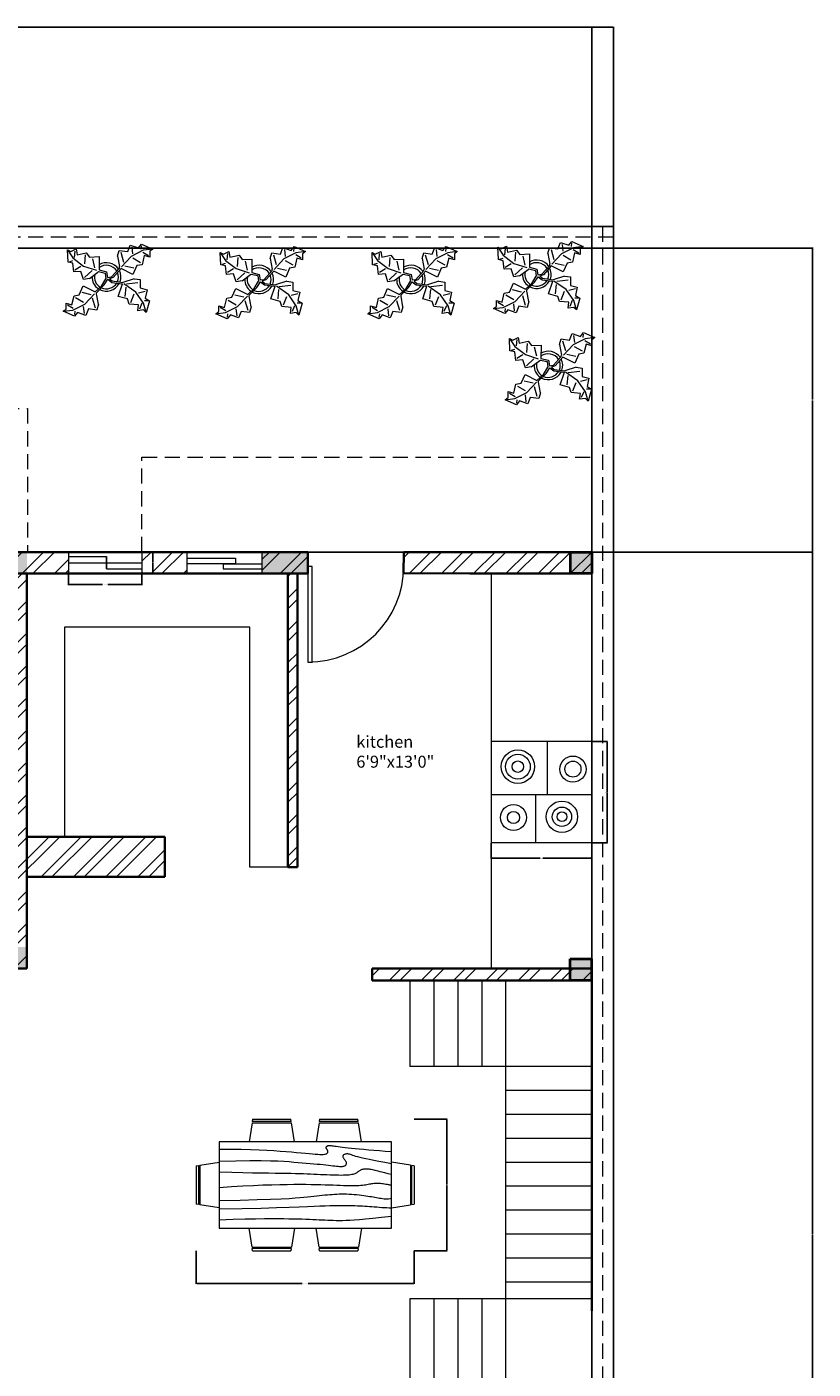
# Model space of a CAD drawing. Units: inches. Extents: x 19613 to 21413, y 12082 to 13202.
# Tile 9 of 9: x 21084 to 21413, y 12641 to 13202. Entities that reach past the tile are written whole.
import ezdxf

# ---------------------------------------------------------------- set-up
doc = ezdxf.new("R2010")
doc.units = ezdxf.units.IN
doc.linetypes.add('HIDDEN', pattern=[9.525, 6.35, -3.175])
for name, color, linetype, lineweight in [('A-ANNO-DIMS', 2, 'Continuous', 18), ('A-AREA-IDEN', 7, 'Continuous', 18), ('A-COLS', 7, 'Continuous', 40), ('A-COLS-PATT', 6, 'Continuous', 13), ('A-DOOR', 3, 'Continuous', 18), ('A-EQPM', 8, 'Continuous', 18), ('A-FLOR-CASE', 9, 'Continuous', 18), ('A-FLOR-HIDN', 8, 'HIDDEN', 13), ('A-FLOR-STRS', 7, 'Continuous', 18), ('A-FURN', 8, 'Continuous', 18), ('A-GLAZ', 4, 'Continuous', 18), ('A-WALL', 7, 'Continuous', 35), ('A-WALL-PATT', 252, 'Continuous', 13), ('C-PROP', 7, 'Continuous', 25), ('C-PROP-HIDN', 8, 'HIDDEN', 13), ('L-PLNT', 116, 'Continuous', 18)]:
    doc.layers.add(name, color=color, linetype=linetype, lineweight=lineweight)
doc.styles.get("Standard").update_dxf_attribs({"font": 'arial.ttf'})
doc.dimstyles.get("Standard").update_dxf_attribs({"dimtxt": 0.18, "dimasz": 0.18, "dimexe": 0.18, "dimexo": 0.0625, "dimgap": 0.09, "dimtad": 0, "dimtih": 1, "dimtoh": 1, "dimdec": 4, "dimzin": 0, "dimdsep": 46, "dimtxsty": 'Standard', "dimcen": 0.09, "dimadec": 0, "dimazin": 0, "dimtfac": 1, "dimtdec": 4, "dimtofl": 0, "dimtmove": 0, "dimatfit": 3, "dimfxl": 1, "dimtolj": 1, "dimtzin": 0, "dimarcsym": 0})

# ---------------------------------------------------------------- blocks, each defined once
blk = doc.blocks.new('*U2')
for p, q in [((0, 0), (0, 6)), ((40, 0), (40, 6))]:
    blk.add_line(p, q)
blk.add_lwpolyline([(0, 0), (0, -40), (1.75, -40), (1.75, 0)], close=True)
blk.add_arc((0, 0), 40, 270, 0)
blk = doc.blocks.new('Dining Set - 36 x 72 in.')
for p, q in [((-22.2343, 26.00059), (-23.4847, 17.99762)), ((-22.2304, 26), (-5.7608, 26)), ((-22, 27.5), (-22.1562, 26.50042)), ((-5.8416, 26.5), (-22.1534, 26.5)), ((-22, 27.5), (-6, 27.5)), ((-5.8437, 26.49966), (-6, 27.5)), ((-4.5152, 17.99762), (-5.7655, 25.99926)), ((5.7657, 26.00059), (4.5153, 17.99762)), ((5.7696, 26), (22.2392, 26)), ((6, 27.5), (5.8438, 26.50042)), ((22.1584, 26.5), (5.8466, 26.5)), ((6, 27.5), (22, 27.5)), ((22.1563, 26.49966), (22, 27.5)), ((23.4848, 17.99762), (22.2345, 25.99926)), ((36, 18), (-36, 18)), ((-36, 18), (-36, -18)), ((36, -18), (36, 18)), ((-45.5, 8), (-44.5004, 8.15617)), ((-45.5, 8), (-45.5, -8)), ((-44.5, -8.15843), (-44.5, 8.15338)), ((-44.0006, 8.23428), (-35.9976, 9.48474)), ((-44, 8.23041), (-44, -8.23915)), ((44.0006, 8.23428), (35.9976, 9.48474)), ((44, 8.23041), (44, -8.23915)), ((44.5, -8.15843), (44.5, 8.15338)), ((45.5, 8), (44.5005, 8.15617)), ((45.5, 8), (45.5, -8)), ((-44.4997, -8.15631), (-45.5, -8)), ((-35.9976, -9.48476), (-43.9993, -8.2345)), ((35.9976, -9.48476), (43.9993, -8.2345)), ((44.4997, -8.15631), (45.5, -8)), ((-36, -18), (36, -18)), ((-22.2343, -26.0006), (-23.4847, -17.99762)), ((-4.5152, -17.99762), (-5.7655, -25.99928)), ((5.7657, -26.0006), (4.5153, -17.99762)), ((23.4848, -17.99762), (22.2345, -25.99928)), ((-22.2304, -26), (-5.7608, -26)), ((-22, -27.5), (-22.1562, -26.50044)), ((-5.8416, -26.5), (-22.1534, -26.5)), ((-22, -27.5), (-6, -27.5)), ((-5.8437, -26.49967), (-6, -27.5)), ((5.7696, -26), (22.2392, -26)), ((6, -27.5), (5.8438, -26.50044)), ((22.1584, -26.5), (5.8466, -26.5)), ((6, -27.5), (22, -27.5)), ((22.1563, -26.49967), (22, -27.5))]:
    blk.add_line(p, q)
for points in [[(-36, 15), (-31.1772, 14.97754), (-26.8079, 14.91406), (-22.8538, 14.81543), (-19.276, 14.6875), (-16.0362, 14.53613), (-13.0957, 14.36718), (-10.4159, 14.18652), (-7.9583, 14), (-5.6904, 13.81315), (-3.6035, 13.63021), (-1.6954, 13.45508), (0.0365, 13.29166), (1.5945, 13.14388), (2.9811, 13.01562), (4.1988, 12.9108), (5.25, 12.83333), (6.1393, 12.78613), (6.8802, 12.76823), (7.4883, 12.77767), (7.9792, 12.8125), (8.3685, 12.87077), (8.6719, 12.95052), (8.9049, 13.0498), (9.0833, 13.16666), (9.2205, 13.29899), (9.3216, 13.44401), (9.3895, 13.59879), (9.4271, 13.76041), (9.4373, 13.92594), (9.4232, 14.09245), (9.3875, 14.257), (9.3333, 14.41666), (9.2638, 14.56917), (9.1836, 14.71484), (9.0975, 14.85465), (9.0104, 14.98958), (8.9272, 15.1206), (8.8529, 15.2487), (8.7922, 15.37483), (8.75, 15.5), (8.7305, 15.62467), (8.7344, 15.74739), (8.7617, 15.86621), (8.8125, 15.97916), (8.8867, 16.08431), (8.9844, 16.17968), (9.1055, 16.26334), (9.25, 16.33333), (9.4189, 16.38802), (9.6172, 16.42708), (9.8506, 16.45052), (10.125, 16.45833), (10.4463, 16.45052), (10.8203, 16.42708), (11.2529, 16.38802), (11.75, 16.33333), (12.3184, 16.26318), (12.9694, 16.17838), (13.7151, 16.07991), (14.5677, 15.96875), (15.5395, 15.84586), (16.6426, 15.71224), (17.8893, 15.56884), (19.2917, 15.41666), (20.859, 15.25667), (22.5879, 15.08984), (24.4721, 14.91715), (26.5052, 14.73958), (28.6809, 14.5581), (30.9929, 14.3737), (33.4347, 14.18733), (36, 14)], [(-36, 10), (-28.9766, 10.14274), (-23.1725, 10.20442), (-18.4241, 10.19775), (-14.5677, 10.13541), (-11.4399, 10.03011), (-8.877, 9.89453), (-6.7154, 9.74137), (-4.7917, 9.58333), (-2.9698, 9.43082), (-1.2246, 9.28515), (0.4415, 9.14534), (2.026, 9.01041), (3.5266, 8.87939), (4.9408, 8.7513), (6.266, 8.62516), (7.5, 8.5), (8.6411, 8.37549), (9.6914, 8.2539), (10.6538, 8.13818), (11.5312, 8.03125), (12.3267, 7.93603), (13.043, 7.85547), (13.6831, 7.79248), (14.25, 7.75), (14.7471, 7.7303), (15.1797, 7.73307), (15.5537, 7.75732), (15.875, 7.80208), (16.1494, 7.86637), (16.3828, 7.94922), (16.5811, 8.04964), (16.75, 8.16666), (16.8944, 8.29915), (17.0143, 8.44531), (17.1089, 8.60319), (17.1771, 8.77083), (17.218, 8.94629), (17.2305, 9.1276), (17.2137, 9.31282), (17.1667, 9.5), (17.0895, 9.6875), (16.987, 9.875), (16.8649, 10.0625), (16.7292, 10.25), (16.5856, 10.4375), (16.4401, 10.625), (16.2985, 10.8125), (16.1667, 11), (16.05, 11.18733), (15.9518, 11.3737), (15.8752, 11.5581), (15.8229, 11.73958), (15.798, 11.91715), (15.8034, 12.08984), (15.842, 12.25667), (15.9167, 12.41666), (16.0295, 12.56836), (16.1784, 12.70833), (16.3605, 12.83268), (16.5729, 12.9375), (16.8127, 13.01888), (17.0768, 13.07291), (17.3625, 13.0957), (17.6667, 13.08333), (17.9894, 13.03312), (18.3418, 12.94726), (18.7382, 12.82918), (19.1927, 12.68229), (19.7195, 12.51001), (20.3327, 12.31575), (21.0465, 12.10294), (21.875, 11.875), (22.8357, 11.63354), (23.959, 11.37304), (25.2786, 11.08618), (26.8282, 10.76562), (28.6414, 10.40405), (30.752, 9.99414), (33.1936, 9.52856), (36, 9)], [(-36, 5.5), (-30.7157, 5.3348), (-26.069, 5.20963), (-21.9946, 5.11767), (-18.4271, 5.05208), (-15.3009, 5.00602), (-12.5508, 4.97265), (-10.1112, 4.94515), (-7.9167, 4.91666), (-5.909, 4.88167), (-4.0586, 4.83984), (-2.3429, 4.79215), (-0.7396, 4.73958), (0.7739, 4.6831), (2.22, 4.6237), (3.6213, 4.56233), (5, 4.5), (6.373, 4.43782), (7.7344, 4.3776), (9.0723, 4.32129), (10.375, 4.27083), (11.6309, 4.22819), (12.8281, 4.19531), (13.9551, 4.17415), (15, 4.16666), (15.954, 4.17448), (16.819, 4.19791), (17.6001, 4.23698), (18.3021, 4.29166), (18.9299, 4.36198), (19.4883, 4.44791), (19.9823, 4.54948), (20.4167, 4.66666), (20.7969, 4.79899), (21.1302, 4.94401), (21.4245, 5.09879), (21.6875, 5.26041), (21.9271, 5.42594), (22.1511, 5.59245), (22.3672, 5.757), (22.5834, 5.91666), (22.8065, 6.06868), (23.0404, 6.21093), (23.2879, 6.34147), (23.5521, 6.45833), (23.8358, 6.55957), (24.142, 6.64323), (24.4735, 6.70735), (24.8334, 6.75), (25.2235, 6.76969), (25.642, 6.76692), (26.0858, 6.74267), (26.5521, 6.69791), (27.0379, 6.63362), (27.5404, 6.55078), (28.0565, 6.45036), (28.5834, 6.33333), (29.1242, 6.19987), (29.7071, 6.04687), (30.3661, 5.87044), (31.1354, 5.66666), (32.0493, 5.43164), (33.142, 5.16146), (34.4475, 4.85221), (36, 4.5)], [(-36, -1), (-30.7915, -0.6591), (-26.0195, -0.38216), (-21.6519, -0.16284), (-17.6563, 0.00521), (-14.0005, 0.12833), (-10.6523, 0.21289), (-7.5796, 0.26522), (-4.75, 0.29166), (-2.134, 0.29793), (0.2878, 0.28711), (2.5317, 0.26163), (4.6146, 0.22396), (6.5529, 0.17651), (8.3633, 0.12174), (10.0623, 0.06209), (11.6667, 0), (13.1899, -0.06201), (14.6341, -0.1211), (15.9982, -0.17432), (17.2813, -0.21875), (18.4823, -0.25147), (19.6003, -0.26953), (20.6343, -0.27002), (21.5834, -0.25), (22.4481, -0.20768), (23.2357, -0.14584), (23.9549, -0.06836), (24.6146, 0.02083), (25.2235, 0.11784), (25.7904, 0.21875), (26.3241, 0.31966), (26.8334, 0.41666), (27.3265, 0.50618), (27.8099, 0.58593), (28.2894, 0.65397), (28.7709, 0.70833), (29.2601, 0.74707), (29.763, 0.76823), (30.2855, 0.76985), (30.8334, 0.75), (31.4088, 0.70784), (31.9994, 0.64713), (32.589, 0.57275), (33.1615, 0.48958), (33.7008, 0.4025), (34.1908, 0.3164), (34.6153, 0.23616), (34.9584, 0.16666), (35.2099, 0.11165), (35.3848, 0.07031), (35.504, 0.04069), (35.5886, 0.02083), (35.6594, 0.00879), (35.7377, 0.0026), (35.8442, 0.00032), (36, 0)], [(-36, -6.5), (-27.1843, -6.31267), (-20.084, -6.1263), (-14.469, -5.9419), (-10.1094, -5.76042), (-6.7752, -5.58285), (-4.2363, -5.41016), (-2.2629, -5.24333), (-0.625, -5.08334), (0.8708, -4.93099), (2.2715, -4.78646), (3.5872, -4.64974), (4.8281, -4.52084), (6.0046, -4.39974), (7.127, -4.28646), (8.2053, -4.18099), (9.25, -4.08334), (10.2705, -3.99382), (11.2734, -3.91407), (12.2647, -3.84603), (13.25, -3.79167), (14.2354, -3.75293), (15.2266, -3.73177), (16.2295, -3.73015), (17.25, -3.75), (18.2912, -3.79248), (19.3451, -3.85547), (20.4009, -3.93604), (21.4479, -4.03125), (22.4754, -4.13819), (23.4727, -4.25391), (24.4289, -4.37549), (25.3334, -4.5), (26.1785, -4.62492), (26.9694, -4.74935), (27.7145, -4.87281), (28.4219, -4.99479), (29.1, -5.11483), (29.7572, -5.23242), (30.4016, -5.34709), (31.0417, -5.45834), (31.6837, -5.56437), (32.3262, -5.65821), (32.9658, -5.73153), (33.599, -5.77604), (34.2224, -5.78345), (34.8327, -5.74545), (35.4264, -5.65373), (36, -5.5)], [(-36, -10), (-26.4022, -9.81299), (-18.4675, -9.62891), (-11.9839, -9.45069), (-6.7396, -9.28125), (-2.5226, -9.12354), (0.8789, -8.98047), (3.6769, -8.85498), (6.0833, -8.75), (8.2767, -8.66765), (10.3021, -8.60677), (12.1712, -8.56543), (13.8958, -8.54167), (15.4876, -8.53353), (16.9583, -8.53907), (18.3197, -8.55632), (19.5834, -8.58334), (20.7616, -8.61841), (21.8685, -8.66081), (22.9188, -8.71004), (23.9271, -8.76563), (24.9081, -8.82707), (25.8763, -8.89388), (26.8465, -8.96558), (27.8334, -9.04167), (28.8474, -9.12118), (29.8828, -9.20117), (30.93, -9.27824), (31.9792, -9.34896), (33.0205, -9.40991), (34.0443, -9.45768), (35.0407, -9.48885), (36, -9.5)], [(-36, -14.5), (-30.0881, -14.33513), (-25.0332, -14.21224), (-20.7312, -14.12647), (-17.0781, -14.07292), (-13.97, -14.04671), (-11.3027, -14.04297), (-8.9724, -14.05681), (-6.875, -14.08334), (-4.9224, -14.11833), (-3.0905, -14.16016), (-1.3709, -14.20785), (0.2448, -14.26042), (1.7647, -14.3169), (3.1973, -14.3763), (4.5507, -14.43767), (5.8333, -14.5), (7.0554, -14.5621), (8.235, -14.62175), (9.3922, -14.67652), (10.5469, -14.72396), (11.7192, -14.76164), (12.929, -14.78711), (14.1965, -14.79794), (15.5417, -14.79167), (16.9933, -14.76424), (18.6152, -14.70508), (20.4804, -14.60197), (22.6615, -14.44271), (25.2312, -14.21509), (28.2624, -13.9069), (31.8277, -13.50594), (36, -13)]]:
    blk.add_lwpolyline(points)
blk = doc.blocks.new('Plant - Rubber or Philodendron')
for p, q in [((-16.2005, 11.4774), (-13.9899, 8.1064)), ((-16.2005, 11.4774), (-14.8639, 10.7964)), ((-16.0159, 6.3329), (-16.2005, 11.4774)), ((-14.8639, 10.7964), (-12.6195, 11.8975)), ((-12.6195, 11.8975), (-12.1909, 9.4345)), ((4.6914, 8.8812), (5.3859, 11.2828)), ((5.3859, 11.2828), (8.8871, 10.7908)), ((8.8871, 10.7908), (9.9809, 13.4933)), ((9.9809, 13.4933), (13.3837, 12.301)), ((15.3859, 11.3055), (10.3916, 8.7942)), ((10.5828, 12.6946), (10.8893, 9.7953)), ((13.3837, 12.301), (14.68, 13.9039)), ((14.5816, 13.2037), (14.3848, 11.8033)), ((14.68, 13.9039), (19.3848, 11.8146)), ((19.3848, 11.8146), (15.3859, 11.3055)), ((19.3848, 11.8146), (18.1868, 10.9119)), ((-14.0069, 5.8704), (-16.0159, 6.3329)), ((-15.3434, 6.5514), (-13.9984, 6.9884)), ((-13.5868, 2.2894), (-14.0069, 5.8704)), ((-13.9899, 8.1064), (-9.5434, 4.7185)), ((-13.3174, 8.325), (-13.0735, 11.0065)), ((-12.1909, 9.4345), (-8.3829, 10.3)), ((-8.8369, 9.409), (-9.0894, 5.6095)), ((-8.3829, 10.3), (-7.0549, 8.501)), ((-7.0549, 8.501), (-3.0284, 8.6941)), ((-4.8529, 4.012), (-5.7184, 7.82)), ((-3.0284, 8.6941), (-3.0709, 3.1041)), ((4.6914, 8.8812), (5.5014, 4.4831)), ((5.9878, 10.4842), (7.1971, 6.3869)), ((10.3916, 8.7942), (6.2847, 4.4028)), ((14.2977, 6.1031), (10.9934, 7.9956)), ((15.7909, 9.1065), (14.8995, 5.3044)), ((15.2875, 10.6053), (17.5907, 9.2105)), ((18.1925, 8.4119), (15.7909, 9.1065)), ((18.1868, 10.9119), (18.1925, 8.4119)), ((-10.6784, 2.491), (-13.5868, 2.2894)), ((-13.1329, 3.1804), (-10.6614, 4.727)), ((-9.5858, -0.8715), (-10.6784, 2.491)), ((-9.5434, 4.7185), (-4.1917, 2.9888)), ((-9.1318, 0.0195), (-5.9793, 2.9025)), ((-7.1228, -0.443), (-3.5248, 2.2131)), ((-3.5248, 2.2131), (-3.3011, 2.4355)), ((-3.3011, 2.4355), (-0.5306, 1.7947)), ((-3.0709, 3.1041), (0.0797, 2.3163)), ((-0.5306, 1.7947), (-0.2255, -0.5527)), ((-0.5306, 1.7947), (-0.5306, 1.7947)), ((0.0797, 2.3163), (0.4866, -0.031)), ((0.4866, -0.031), (2.1141, 0.2298)), ((2.1141, 0.2298), (5.4346, 3.9146)), ((6.1032, 3.6844), (2.8262, -0.031)), ((5.4346, 3.9146), (5.5014, 4.4831)), ((11.1089, 1.1958), (6.1032, 3.6844)), ((7.7005, 4.8881), (11.5025, 3.9967)), ((12.7005, 4.8994), (11.1089, 1.1958)), ((14.8995, 5.3044), (12.7005, 4.8994)), ((-11.3237, -7.2629), (-9.7321, -3.5593)), ((-9.7321, -3.5593), (-4.7264, -6.0479)), ((-7.1228, -0.443), (-9.5858, -0.8715)), ((-2.019, -3.6148), (-4.7264, -6.0479)), ((-4.0579, -6.2781), (-0.9375, -3.1608)), ((-2.019, -3.6148), (-0.2255, -0.5527)), ((-0.9375, -3.1608), (0.5883, -0.8135)), ((0.5883, -0.8135), (2.2447, -2.0916)), ((2.8262, -0.031), (1.3003, -0.5527)), ((1.3003, -0.5527), (2.4193, -1.4655)), ((2.2447, -2.0916), (6.7108, -2.6626)), ((2.4193, -1.4655), (6.895, -2.1175)), ((4.943, -7.9659), (6.7108, -2.6626)), ((11.6605, -0.5413), (6.895, -2.1175)), ((12.3677, -6.1981), (7.219, -2.6772)), ((8.125, -4.0768), (7.7715, -7.9659)), ((8.3544, -2.7453), (13.1973, -2.1704)), ((11.6605, -0.5413), (14.1354, -0.8948)), ((14.1354, -0.8948), (14.1354, -4.4304)), ((14.1354, -4.4304), (16.9638, -5.1375)), ((16.9638, -5.1375), (16.2567, -8.673)), ((-16.8157, -10.7754), (-14.4141, -11.4699)), ((-16.8101, -13.2754), (-16.8157, -10.7754)), ((-14.4141, -11.4699), (-13.5228, -7.6679)), ((-14.0091, -13.669), (-9.0148, -11.1577)), ((-13.5228, -7.6679), (-11.3237, -7.2629)), ((-12.921, -8.4665), (-9.6166, -10.359)), ((-6.3237, -7.2516), (-10.1257, -6.3602)), ((-9.0148, -11.1577), (-4.9047, -6.8122)), ((-4.611, -12.8477), (-5.8203, -8.7504)), ((-4.1246, -6.8466), (-4.0579, -6.2781)), ((-3.3146, -11.2447), (-4.1246, -6.8466)), ((8.8321, -9.0266), (4.943, -7.9659)), ((9.5392, -11.1479), (8.8321, -9.0266)), ((13.4283, -11.5015), (9.5392, -11.1479)), ((10.2463, -10.4408), (11.6605, -6.9053)), ((15.5496, -10.7943), (12.3677, -6.1981)), ((16.2567, -5.8446), (13.4283, -6.5517)), ((14.8425, -10.7943), (13.7819, -13.2692)), ((16.6103, -14.6834), (15.5496, -10.7943)), ((17.3174, -9.7337), (15.9032, -9.7337)), ((16.2567, -8.673), (18.0245, -9.7337)), ((18.0245, -9.7337), (16.6103, -14.6834)), ((-18.008, -14.1781), (-16.8101, -13.2754)), ((-18.008, -14.1781), (-14.0091, -13.669)), ((-13.3032, -16.2674), (-18.008, -14.1781)), ((-13.9107, -12.9688), (-16.2139, -11.574)), ((-12.0069, -14.6645), (-13.3032, -16.2674)), ((-13.2048, -15.5672), (-13.008, -14.1668)), ((-8.6042, -15.8568), (-12.0069, -14.6645)), ((-9.206, -15.0581), (-9.5126, -12.1588)), ((-7.5103, -13.1543), (-8.6042, -15.8568)), ((-4.0092, -13.6463), (-7.5103, -13.1543)), ((-3.3146, -11.2447), (-4.0092, -13.6463)), ((13.0748, -13.9763), (13.4283, -11.5015)), ((15.5496, -13.6228), (13.0748, -13.9763)), ((16.6103, -14.6834), (15.5496, -13.6228))]:
    blk.add_line(p, q)
for centre, radius, start, end in [((0, 0), 6.1275, 34.37569, 120.1028), ((0.0308, 0.1664), 6, 178.6147, 235.1169), ((0.0308, 0.1664), 5, 168.1647, 238.6725), ((-0.0601, -0.2075), 5.2461, 33.82192, 124.9414), ((-0.2664, 0.1682), 5.2775, 338.4094, 20.03007), ((-0.098, 0.1364), 6.1288, 341.2017, 26.09184), ((-0.0234, 0.3825), 6.1492, 242.5812, 331.2714), ((-0.1102, 0.4886), 5.2883, 247.3711, 327.472)]:
    blk.add_arc(centre, radius, start, end)
blk = doc.blocks.new('COL-9x9')
for p, q in [((0, 9), (9, 9)), ((0, 0), (0, 9)), ((9, 9), (9, 0)), ((9, 0), (0, 0))]:
    blk.add_line(p, q)
blk = doc.blocks.new('RANGE-4-BURNER')
for p, q in [((42, 42.44), (0, 42.44)), ((23.29, 42.44), (23.29, 20.04)), ((42, 20.04), (0, 20.04)), ((18.54, 20.04), (18.54, 0)), ((42, 0), (0, 0))]:
    blk.add_line(p, q)
for centre, radius in [((11.11, 31.86), 6.98), ((11.11, 31.86), 5.19), ((11.11, 31.86), 2.41), ((34.12, 30.84), 5.47), ((34.12, 30.84), 3.36), ((34.12, 30.84), 3.36), ((34.12, 30.84), 3.36), ((29.52, 10.94), 6.53), ((29.52, 10.94), 6.53), ((29.52, 10.94), 6.53), ((9.27, 10.62), 5.42), ((9.27, 10.62), 2.53), ((29.52, 10.94), 4.03), ((29.52, 10.94), 2.04)]:
    blk.add_circle(centre, radius)
blk = doc.blocks.new('WINDOW-SHORT-SLIDER-A')
for p, q in [((0, 9), (0, 0)), ((0, 7.09), (15.83, 7.09)), ((15.83, 4.5), (15.83, 7.09)), ((15.83, 7.09), (15.83, 4.5)), ((30.64, 9), (30.64, 0)), ((0, 4.5), (15.83, 4.5)), ((15.83, 4.5), (15.83, 2.04)), ((15.83, 2.04), (15.83, 4.5)), ((15.83, 4.5), (30.64, 4.5)), ((15.83, 2.04), (30.64, 2.04))]:
    blk.add_line(p, q)
blk = doc.blocks.new('WINDOW-SHORT-SLIDER-B')
for p, q in [((0, 9), (0, 0)), ((0, 6.5), (20.33, 6.5)), ((20.33, 6.5), (20.33, 4.13)), ((31.36, 9), (31.36, 0)), ((20.33, 4.13), (0, 4.13)), ((15.2, 4.13), (15.2, 1.96)), ((15.2, 4.13), (31.36, 4.13)), ((15.2, 1.96), (31.36, 1.96))]:
    blk.add_line(p, q)
blk = doc.blocks.new('STAIR-RETURN-FLIGHT')
for p, q in [((0, 169), (0, 133)), ((10, 169), (10, 133)), ((20, 169), (20, 133)), ((30, 169), (30, 133)), ((76, 169), (40, 169)), ((76, 169), (40, 169)), ((40, 169), (40, 0)), ((76, 169), (76, 133)), ((76, 169), (76, 133)), ((76, 133), (0, 133)), ((76, 123), (40, 123)), ((76, 113), (40, 113)), ((76, 103), (40, 103)), ((76, 93), (40, 93)), ((76, 83), (40, 83)), ((76, 73), (40, 73)), ((76, 63), (40, 63)), ((76, 31), (76, 67)), ((76, 53), (40, 53)), ((76, 43), (40, 43)), ((76, 36), (0, 36)), ((0, 36), (0, 0)), ((10, 36), (10, 0)), ((20, 36), (20, 0)), ((30, 36), (30, 0)), ((76, 0), (76, 36))]:
    blk.add_line(p, q)
blk = doc.blocks.new('*D51')
at = {"layer": 'A-ANNO-DIMS', "color": 0, "lineweight": -2, "transparency": 16777216}
for p, q in [((21155.23, 12690.27), (21155.23, 12676.5)), ((21246.23, 12690.27), (21246.23, 12676.5)), ((21155.41, 12676.68), (21199.45, 12676.68)), ((21246.05, 12676.68), (21202.01, 12676.68))]:
    blk.add_line(p, q, dxfattribs=at)
at = {"layer": 'A-ANNO-DIMS', "color": 0, "transparency": 16777216}
for points in [[(21155.41, 12676.71), (21155.41, 12676.65), (21155.23, 12676.68)], [(21246.05, 12676.71), (21246.05, 12676.65), (21246.23, 12676.68)]]:
    blk.add_solid(points, dxfattribs=at)
at = {"layer": 'Defpoints', "color": 0, "transparency": 16777216}
for p in [(21155.23, 12690.33), (21246.23, 12690.33), (21246.23, 12676.68)]:
    blk.add_point(p, dxfattribs=at)
at = {"layer": 'A-ANNO-DIMS', "color": 0, "transparency": 16777216, "insert": (21200.73, 12676.68), "char_height": 0.18, "attachment_point": 5}
blk.add_mtext('\\A1;DINING SET 91 TYP.', dxfattribs=at)
blk = doc.blocks.new('*D52')
at = {"layer": 'A-ANNO-DIMS', "color": 0, "lineweight": -2, "transparency": 16777216}
for p, q in [((21246.29, 12745.33), (21260.06, 12745.33)), ((21259.88, 12745.15), (21259.88, 12718.01)), ((21259.88, 12690.51), (21259.88, 12717.65)), ((21246.29, 12690.33), (21260.06, 12690.33))]:
    blk.add_line(p, q, dxfattribs=at)
at = {"layer": 'A-ANNO-DIMS', "color": 0, "transparency": 16777216}
for points in [[(21259.85, 12745.15), (21259.91, 12745.15), (21259.88, 12745.33)], [(21259.85, 12690.51), (21259.91, 12690.51), (21259.88, 12690.33)]]:
    blk.add_solid(points, dxfattribs=at)
at = {"layer": 'Defpoints', "color": 0, "transparency": 16777216}
for p in [(21246.23, 12745.33), (21259.88, 12745.33), (21246.23, 12690.33)]:
    blk.add_point(p, dxfattribs=at)
at = {"layer": 'A-ANNO-DIMS', "color": 0, "transparency": 16777216, "insert": (21259.88, 12717.83), "char_height": 0.18, "attachment_point": 5}
blk.add_mtext('\\A1;55 TYP.', dxfattribs=at)
blk = doc.blocks.new('*D53')
at = {"layer": 'A-ANNO-DIMS', "color": 0, "lineweight": -2, "transparency": 16777216}
for p, q in [((21320.5, 12903.18), (21326.98, 12903.18)), ((21326.8, 12903), (21326.8, 12882.15)), ((21326.8, 12860.92), (21326.8, 12881.78)), ((21320.5, 12860.74), (21326.98, 12860.74))]:
    blk.add_line(p, q, dxfattribs=at)
at = {"layer": 'A-ANNO-DIMS', "color": 0, "transparency": 16777216}
for points in [[(21326.77, 12903), (21326.83, 12903), (21326.8, 12903.18)], [(21326.77, 12860.92), (21326.83, 12860.92), (21326.8, 12860.74)]]:
    blk.add_solid(points, dxfattribs=at)
at = {"layer": 'Defpoints', "color": 0, "transparency": 16777216}
for p in [(21320.43, 12903.18), (21326.8, 12903.18), (21320.43, 12860.74)]:
    blk.add_point(p, dxfattribs=at)
at = {"layer": 'A-ANNO-DIMS', "color": 0, "transparency": 16777216, "insert": (21326.8, 12881.96), "char_height": 0.18, "attachment_point": 5}
blk.add_mtext('\\A1;RANGE 42 TYP.', dxfattribs=at)
blk = doc.blocks.new('*D54')
at = {"layer": 'A-ANNO-DIMS', "color": 0, "lineweight": -2, "transparency": 16777216}
for p, q in [((21278.43, 12860.68), (21278.43, 12854.2)), ((21320.43, 12860.68), (21320.43, 12854.2)), ((21278.61, 12854.38), (21298.9, 12854.38)), ((21320.25, 12854.38), (21299.97, 12854.38))]:
    blk.add_line(p, q, dxfattribs=at)
at = {"layer": 'A-ANNO-DIMS', "color": 0, "transparency": 16777216}
for points in [[(21278.61, 12854.41), (21278.61, 12854.35), (21278.43, 12854.38)], [(21320.25, 12854.41), (21320.25, 12854.35), (21320.43, 12854.38)]]:
    blk.add_solid(points, dxfattribs=at)
at = {"layer": 'Defpoints', "color": 0, "transparency": 16777216}
for p in [(21278.43, 12860.74), (21320.43, 12860.74), (21320.43, 12854.38)]:
    blk.add_point(p, dxfattribs=at)
at = {"layer": 'A-ANNO-DIMS', "color": 0, "transparency": 16777216, "insert": (21299.43, 12854.38), "char_height": 0.18, "attachment_point": 5}
blk.add_mtext('\\A1;42 TYP.', dxfattribs=at)
blk = doc.blocks.new('*D65')
at = {"layer": 'A-ANNO-DIMS', "color": 0, "lineweight": -2, "transparency": 16777216}
for p, q in [((21101.85, 12973.22), (21101.85, 12968.5)), ((21132.49, 12973.22), (21132.49, 12968.5)), ((21102.03, 12968.68), (21116.03, 12968.68)), ((21132.31, 12968.68), (21118.3, 12968.68))]:
    blk.add_line(p, q, dxfattribs=at)
at = {"layer": 'A-ANNO-DIMS', "color": 0, "transparency": 16777216}
for points in [[(21102.03, 12968.71), (21102.03, 12968.65), (21101.85, 12968.68)], [(21132.31, 12968.71), (21132.31, 12968.65), (21132.49, 12968.68)]]:
    blk.add_solid(points, dxfattribs=at)
at = {"layer": 'Defpoints', "color": 0, "transparency": 16777216}
for p in [(21101.85, 12973.28), (21132.49, 12973.28), (21132.49, 12968.68)]:
    blk.add_point(p, dxfattribs=at)
at = {"layer": 'A-ANNO-DIMS', "color": 0, "transparency": 16777216, "insert": (21117.17, 12968.68), "char_height": 0.18, "attachment_point": 5}
blk.add_mtext('\\A1;SLIDER A 31 TYP.', dxfattribs=at)
blk = doc.blocks.new('*D66')
at = {"layer": 'A-ANNO-DIMS', "color": 0, "lineweight": -2, "transparency": 16777216}
for p, q in [((21132.55, 12982.28), (21137.26, 12982.28)), ((21137.08, 12982.1), (21137.08, 12977.96)), ((21132.55, 12973.28), (21137.26, 12973.28)), ((21137.08, 12973.46), (21137.08, 12977.6))]:
    blk.add_line(p, q, dxfattribs=at)
at = {"layer": 'A-ANNO-DIMS', "color": 0, "transparency": 16777216}
for points in [[(21137.05, 12982.1), (21137.11, 12982.1), (21137.08, 12982.28)], [(21137.05, 12973.46), (21137.11, 12973.46), (21137.08, 12973.28)]]:
    blk.add_solid(points, dxfattribs=at)
at = {"layer": 'Defpoints', "color": 0, "transparency": 16777216}
for p in [(21132.49, 12982.28), (21137.08, 12982.28), (21132.49, 12973.28)]:
    blk.add_point(p, dxfattribs=at)
at = {"layer": 'A-ANNO-DIMS', "color": 0, "transparency": 16777216, "insert": (21137.08, 12977.78), "char_height": 0.18, "attachment_point": 5}
blk.add_mtext('\\A1;9 TYP.', dxfattribs=at)
blk = doc.blocks.new('*D85')
at = {"layer": 'A-ANNO-DIMS', "color": 0, "lineweight": -2, "transparency": 16777216}
for p, q in [((20798.43, 13118.34), (20798.43, 13201.71)), ((20798.61, 13201.53), (21063.66, 13201.53)), ((21329.25, 13201.53), (21064.21, 13201.53)), ((21329.43, 13118.34), (21329.43, 13201.71))]:
    blk.add_line(p, q, dxfattribs=at)
at = {"layer": 'A-ANNO-DIMS', "color": 0, "transparency": 16777216}
for points in [[(20798.61, 13201.56), (20798.61, 13201.5), (20798.43, 13201.53)], [(21329.25, 13201.56), (21329.25, 13201.5), (21329.43, 13201.53)]]:
    blk.add_solid(points, dxfattribs=at)
at = {"layer": 'Defpoints', "color": 0, "transparency": 16777216}
for p in [(21329.43, 13201.53), (20798.43, 13118.28), (21329.43, 13118.28)]:
    blk.add_point(p, dxfattribs=at)
at = {"layer": 'A-ANNO-DIMS', "color": 0, "transparency": 16777216, "insert": (21063.93, 13201.53), "char_height": 0.18, "attachment_point": 5}
blk.add_mtext('\\A1;531', dxfattribs=at)
blk = doc.blocks.new('*D86')
at = {"layer": 'A-ANNO-DIMS', "color": 0, "lineweight": -2, "transparency": 16777216}
for p, q in [((21320.5, 13109.28), (21412.86, 13109.28)), ((21412.68, 13109.1), (21412.68, 13045.96)), ((21412.68, 12982.46), (21412.68, 13045.6)), ((21320.5, 12982.28), (21412.86, 12982.28))]:
    blk.add_line(p, q, dxfattribs=at)
at = {"layer": 'A-ANNO-DIMS', "color": 0, "transparency": 16777216}
for points in [[(21412.65, 13109.1), (21412.71, 13109.1), (21412.68, 13109.28)], [(21412.65, 12982.46), (21412.71, 12982.46), (21412.68, 12982.28)]]:
    blk.add_solid(points, dxfattribs=at)
at = {"layer": 'Defpoints', "color": 0, "transparency": 16777216}
for p in [(21320.43, 13109.28), (21412.68, 13109.28), (21320.43, 12982.28)]:
    blk.add_point(p, dxfattribs=at)
at = {"layer": 'A-ANNO-DIMS', "color": 0, "transparency": 16777216, "insert": (21412.68, 13045.78), "char_height": 0.18, "attachment_point": 5}
blk.add_mtext('\\A1;127', dxfattribs=at)
blk = doc.blocks.new('*D87')
at = {"layer": 'A-ANNO-DIMS', "color": 0, "lineweight": -2, "transparency": 16777216}
for p, q in [((20218.76, 12982.28), (21412.86, 12982.28)), ((21412.68, 12982.1), (21412.68, 12697.46)), ((21412.68, 12412.46), (21412.68, 12697.1)), ((20218.76, 12412.28), (21412.86, 12412.28))]:
    blk.add_line(p, q, dxfattribs=at)
at = {"layer": 'A-ANNO-DIMS', "color": 0, "transparency": 16777216}
for points in [[(21412.65, 12982.1), (21412.71, 12982.1), (21412.68, 12982.28)], [(21412.65, 12412.46), (21412.71, 12412.46), (21412.68, 12412.28)]]:
    blk.add_solid(points, dxfattribs=at)
at = {"layer": 'Defpoints', "color": 0, "transparency": 16777216}
for p in [(20218.69, 12982.28), (21412.68, 12982.28), (20218.69, 12412.28)]:
    blk.add_point(p, dxfattribs=at)
at = {"layer": 'A-ANNO-DIMS', "color": 0, "transparency": 16777216, "insert": (21412.68, 12697.28), "char_height": 0.18, "attachment_point": 5}
blk.add_mtext('\\A1;570', dxfattribs=at)
blk = doc.blocks.new('*D98')
at = {"layer": 'A-ANNO-DIMS', "color": 0, "lineweight": -2, "transparency": 16777216}
for p, q in [((20807.43, 12982.34), (20807.43, 13201.71)), ((20807.61, 13201.53), (21063.64, 13201.53)), ((21320.25, 13201.53), (21064.22, 13201.53)), ((21320.43, 12982.34), (21320.43, 13201.71))]:
    blk.add_line(p, q, dxfattribs=at)
at = {"layer": 'A-ANNO-DIMS', "color": 0, "transparency": 16777216}
for points in [[(20807.61, 13201.56), (20807.61, 13201.5), (20807.43, 13201.53)], [(21320.25, 13201.56), (21320.25, 13201.5), (21320.43, 13201.53)]]:
    blk.add_solid(points, dxfattribs=at)
at = {"layer": 'Defpoints', "color": 0, "transparency": 16777216}
for p in [(21320.43, 13201.53), (20807.43, 12982.28), (21320.43, 12982.28)]:
    blk.add_point(p, dxfattribs=at)
at = {"layer": 'A-ANNO-DIMS', "color": 0, "transparency": 16777216, "insert": (21063.93, 13201.53), "char_height": 0.18, "attachment_point": 5}
blk.add_mtext('\\A1;513', dxfattribs=at)
blk = doc.blocks.new('*D99')
at = {"layer": 'A-ANNO-DIMS', "color": 0, "lineweight": -2, "transparency": 16777216}
for p, q in [((21320.5, 12982.28), (21412.86, 12982.28)), ((21412.68, 12982.1), (21412.68, 12697.46)), ((21412.68, 12412.46), (21412.68, 12697.1)), ((21320.5, 12412.28), (21412.86, 12412.28))]:
    blk.add_line(p, q, dxfattribs=at)
at = {"layer": 'A-ANNO-DIMS', "color": 0, "transparency": 16777216}
for points in [[(21412.65, 12982.1), (21412.71, 12982.1), (21412.68, 12982.28)], [(21412.65, 12412.46), (21412.71, 12412.46), (21412.68, 12412.28)]]:
    blk.add_solid(points, dxfattribs=at)
at = {"layer": 'Defpoints', "color": 0, "transparency": 16777216}
for p in [(21320.43, 12982.28), (21412.68, 12982.28), (21320.43, 12412.28)]:
    blk.add_point(p, dxfattribs=at)
at = {"layer": 'A-ANNO-DIMS', "color": 0, "transparency": 16777216, "insert": (21412.68, 12697.28), "char_height": 0.18, "attachment_point": 5}
blk.add_mtext('\\A1;570', dxfattribs=at)

msp = doc.modelspace()

# ---------------------------------------------------------------- hatches: boundary and pattern name
at = {"layer": 'A-COLS-PATT'}
h = msp.add_hatch(color=256, dxfattribs=at)
h.dxf.hatch_style = 1
h.paths.add_polyline_path([(20816.4328, 12982.279), (20807.4339, 12982.279), (20807.4339, 12973.279), (20816.4328, 12973.279)])
h.paths.add_polyline_path([(21084.4339, 12982.279), (21075.4339, 12982.279), (21075.4339, 12973.279), (21084.4339, 12973.279)])
h.paths.add_polyline_path([(21320.4339, 12982.279), (21311.4729, 12982.279), (21311.4729, 12973.279), (21320.4339, 12973.279)])
h.paths.add_polyline_path([(21320.3201, 12808.279), (21311.3201, 12808.279), (21311.3201, 12803.279), (21320.3201, 12803.279)])
h.paths.add_polyline_path([(21320.3201, 12812.279), (21311.3201, 12812.279), (21311.3201, 12808.279), (21320.3201, 12808.279)])
h.paths.add_polyline_path([(21320.3574, 12634.279), (21311.3574, 12634.279), (21311.3574, 12625.279), (21320.3574, 12625.279)])
h.paths.add_polyline_path([(21319.9035, 12421.1076), (21310.9035, 12421.1076), (21310.9035, 12412.279), (21319.9035, 12412.279)])
h.paths.add_polyline_path([(21086.1238, 12454.2407), (21077.1238, 12454.2407), (21077.1238, 12445.279), (21077.4339, 12445.279), (21086.1238, 12445.279)])
h.paths.add_polyline_path([(21014.4339, 12454.2407), (21005.4339, 12454.2407), (21005.4339, 12445.279), (21014.4339, 12445.279)])
h.paths.add_polyline_path([(21014.3637, 12634.279), (21005.3637, 12634.279), (21005.3637, 12625.5213), (21014.3637, 12625.5213)])
h.paths.add_polyline_path([(21086.4339, 12634.279), (21077.4339, 12634.279), (21077.4339, 12625.5213), (21086.4339, 12625.5213)])
h.paths.add_polyline_path([(20814.1423, 12634.279), (20807.4339, 12634.279), (20807.4339, 12625.4792), (20814.1423, 12625.4792)])
h.paths.add_polyline_path([(20807.4339, 12634.279), (20807.4339, 12634.4792), (20805.1423, 12634.4792), (20805.1423, 12625.4792), (20807.4339, 12625.4792)])
h.paths.add_polyline_path([(20807.4339, 12439.1296), (20802.9339, 12439.1296), (20802.9339, 12430.1296), (20807.4339, 12430.1296)])
h.paths.add_polyline_path([(20802.9339, 12439.1296), (20798.4339, 12439.1296), (20798.4339, 12430.1296), (20802.9339, 12430.1296)])
h.paths.add_polyline_path([(20813.4646, 12817.279), (20807.4339, 12817.279), (20807.4339, 12808.279), (20813.4646, 12808.279)])
h.paths.add_polyline_path([(20807.4339, 12817.279), (20804.4646, 12817.279), (20804.4646, 12808.279), (20807.4339, 12808.279)])
h.paths.add_polyline_path([(20896.8418, 12817.279), (20887.8418, 12817.279), (20887.8418, 12808.279), (20896.8418, 12808.279)])
h.paths.add_polyline_path([(21084.4339, 12817.279), (21075.4339, 12817.279), (21075.4339, 12808.279), (21084.4339, 12808.279)])
h.paths.add_polyline_path([(21201.8616, 12982.279), (21182.5788, 12982.279), (21182.5788, 12973.279), (21193.4339, 12973.279), (21201.8616, 12973.279), (21201.8616, 12976.279)])
at = {"layer": 'A-WALL-PATT'}
h = msp.add_hatch(dxfattribs=at)
h.set_pattern_fill('ANSI32', color=256)
h.paths.add_polyline_path([(20223.1937, 13118.279), (20218.6937, 13118.279), (19701.1937, 13118.279), (19701.1937, 13113.779), (20223.1937, 13113.779)])
h.paths.add_polyline_path([(19849.7315, 12982.279), (19799.9854, 12982.279), (19799.9854, 12973.279), (19849.7315, 12973.279)])
h.paths.add_polyline_path([(19755.5378, 12982.279), (19705.6937, 12982.279), (19705.6937, 12973.279), (19755.5378, 12973.279)])
h.paths.add_polyline_path([(20000.1054, 12982.279), (19950.0534, 12982.279), (19950.0534, 12974.1171), (19950.0534, 12973.279), (20000.1054, 12973.279)])
h.paths.add_polyline_path([(20049.4797, 12982.279), (20030.7476, 12982.279), (20030.7476, 12973.279), (20049.4797, 12973.279)])
h.paths.add_polyline_path([(20100.1214, 12982.279), (20080.8386, 12982.279), (20080.8386, 12973.279), (20100.1214, 12973.279), (20100.1214, 12976.279)])
h.paths.add_polyline_path([(20218.6937, 12982.279), (20167.6937, 12982.279), (20140.1214, 12982.279), (20140.1214, 12976.279, -0.01769781), (20140.0212, 12973.45), (20167.6937, 12973.279), (20176.6937, 12973.279), (20218.6937, 12973.279)])
h.paths.add_polyline_path([(19851.5503, 12814.279), (19851.5503, 12817.279), (19793.6937, 12817.279), (19789.6937, 12817.279), (19705.6937, 12817.279), (19705.6937, 12808.279), (19851.5503, 12808.279)])
h.paths.add_polyline_path([(19982.6937, 12973.279), (19973.6937, 12973.279), (19973.6937, 12817.279), (19887.5503, 12817.279), (19887.5503, 12808.279), (19973.6937, 12808.279), (19982.6937, 12808.279)])
h.paths.add_polyline_path([(20058.6937, 12850.5529), (19982.6937, 12850.5529), (19982.6937, 12846.5529), (20058.6937, 12846.5529)])
h.paths.add_polyline_path([(20095.6937, 12973.279), (20091.6937, 12973.279), (20091.6937, 12850.5529), (20087.6937, 12850.5529), (20087.6937, 12846.5529), (20095.6937, 12846.5529)])
h.paths.add_polyline_path([(20218.6937, 12808.279), (20140.8605, 12808.279), (20126.9413, 12808.279), (20126.9413, 12803.279), (20140.8605, 12803.279), (20218.6937, 12803.279)])
h.paths.add_polyline_path([(19738.3931, 12634.279), (19705.6937, 12634.279), (19705.6937, 12625.279), (19738.3931, 12625.279)])
h.paths.add_polyline_path([(19912.6937, 12634.279), (19903.6937, 12634.279), (19891.5503, 12634.279), (19891.5503, 12625.279), (19903.6937, 12625.279), (19903.6937, 12445.279), (19975.6937, 12445.279), (20128.6937, 12445.279), (20128.6937, 12412.279), (20149.8479, 12412.279), (20149.8479, 12421.279), (20137.6937, 12421.279), (20137.6937, 12454.279), (20137.6937, 12580.2801), (20133.6937, 12580.2801), (20133.6937, 12454.279), (19984.6937, 12454.279), (19984.6937, 12625.279), (19993.6937, 12625.279), (19993.6937, 12634.279), (19984.6937, 12634.279), (19975.6937, 12634.279), (19975.6937, 12454.279), (19912.6937, 12454.279)])
h.paths.add_polyline_path([(20218.6937, 12634.279), (20137.6937, 12634.279), (20029.6937, 12634.279), (20029.6937, 12625.279), (20137.6937, 12625.279), (20218.6937, 12625.279)])
h.paths.add_polyline_path([(21014.4339, 12634.279), (21005.4339, 12634.279), (20993.2905, 12634.279), (20993.2905, 12625.279), (21005.4339, 12625.279), (21005.4339, 12445.279), (21077.4339, 12445.279), (21230.4339, 12445.279), (21230.4339, 12412.279), (21251.5881, 12412.279), (21251.5881, 12421.279), (21239.4339, 12421.279), (21239.4339, 12454.279), (21239.4339, 12580.2801), (21235.4339, 12580.2801), (21235.4339, 12454.279), (21086.4339, 12454.279), (21086.4339, 12625.279), (21095.4339, 12625.279), (21095.4339, 12634.279), (21086.4339, 12634.279), (21077.4339, 12634.279), (21077.4339, 12454.279), (21014.4339, 12454.279)])
h.paths.add_polyline_path([(20840.1333, 12634.279), (20807.4339, 12634.279), (20807.4339, 12625.279), (20840.1333, 12625.279)])
h.paths.add_polyline_path([(20953.2905, 12631.279), (20953.2905, 12634.279), (20930.6216, 12634.279), (20930.6216, 12625.279), (20953.2905, 12625.279)])
h.paths.add_polyline_path([(21320.4339, 12634.279), (21239.4339, 12634.279), (21131.4339, 12634.279), (21131.4339, 12625.279), (21239.4339, 12625.279), (21320.4339, 12625.279)])
h.paths.add_polyline_path([(21084.4339, 12973.279), (21075.4339, 12973.279), (21075.4339, 12817.279), (20989.2905, 12817.279), (20989.2905, 12808.279), (21075.4339, 12808.279), (21084.4339, 12808.279)])
h.paths.add_polyline_path([(21142.1261, 12863.2893), (21084.4339, 12863.2893), (21084.4339, 12846.5529), (21142.1261, 12846.5529)])
h.paths.add_polyline_path([(21320.4339, 12808.279), (21242.6007, 12808.279), (21228.6815, 12808.279), (21228.6815, 12803.279), (21242.6007, 12803.279), (21320.4339, 12803.279)])
h.paths.add_polyline_path([(20857.278, 12982.279), (20807.4339, 12982.279), (20807.4339, 12973.279), (20857.278, 12973.279)])
h.paths.add_polyline_path([(20951.4717, 12982.279), (20901.7255, 12982.279), (20901.7255, 12973.279), (20951.4717, 12973.279)])
h.paths.add_polyline_path([(21101.8455, 12982.279), (21051.7936, 12982.279), (21051.7936, 12974.1171), (21051.7936, 12973.279), (21101.8455, 12973.279)])
h.paths.add_polyline_path([(21151.2199, 12982.279), (21132.4878, 12982.279), (21132.4878, 12973.279), (21151.2199, 12973.279)])
h.paths.add_polyline_path([(21201.8616, 12982.279), (21182.5788, 12982.279), (21182.5788, 12973.279), (21193.4339, 12973.279), (21201.8616, 12973.279), (21201.8616, 12976.279)])
h.paths.add_polyline_path([(21320.4339, 12982.279), (21269.4339, 12982.279), (21241.8616, 12982.279), (21241.8616, 12976.279, -0.01769781), (21241.7614, 12973.45), (21269.4339, 12973.279), (21278.4339, 12973.279), (21320.4339, 12973.279)])
h.paths.add_polyline_path([(20953.2905, 12817.279), (20895.4339, 12817.279), (20891.4339, 12817.279), (20807.4339, 12817.279), (20807.4339, 12808.279), (20953.2905, 12808.279)])
h.paths.add_polyline_path([(21197.4339, 12973.279), (21193.4339, 12973.279), (21193.4339, 12850.5529), (21197.4339, 12850.5529)])
h.paths.add_polyline_path([(21320.4339, 12550.279), (21272.5278, 12550.279), (21272.5278, 12546.279), (21320.4339, 12546.279)])
h.paths.add_polyline_path([(21320.4339, 12421.279), (21283.2222, 12421.279), (21283.2222, 12412.279), (21320.4339, 12412.279)])

# ---------------------------------------------------------------- linework, layer by layer
at = {"layer": 'A-FLOR-CASE'}
for p, q in [((21278.4339, 12973.279), (21278.4339, 12808.279)), ((21177.5461, 12950.8286), (21100.1645, 12950.8286)), ((21100.1645, 12950.8286), (21100.1645, 12863.2893)), ((21177.5461, 12850.5529), (21177.5461, 12950.8286)), ((21193.4339, 12850.5529), (21177.5461, 12850.5529)), ((21278.4339, 12808.279), (21320.4339, 12808.279))]:
    msp.add_line(p, q, dxfattribs=at)
at = {"layer": 'A-FLOR-HIDN'}
for p, q in [((20912.9732, 13042.279), (21084.6981, 13042.279)), ((21084.6981, 13042.279), (21084.6981, 12982.279)), ((21132.4878, 12982.279), (21132.4878, 13021.8552)), ((21132.4878, 13021.8552), (21320.4339, 13021.8552))]:
    msp.add_line(p, q, dxfattribs=at)
at = {"layer": 'A-WALL'}
for p, q in [((21201.8616, 12982.279), (20901.7255, 12982.279)), ((21201.8616, 12973.279), (21201.8616, 12982.279)), ((21241.7614, 12973.45), (21241.8616, 12982.279)), ((21269.4339, 12982.279), (21241.8616, 12982.279)), ((21320.4339, 12982.279), (21269.4339, 12982.279)), ((21201.8616, 12973.279), (20901.7255, 12973.279)), ((21075.4339, 12973.279), (21084.4339, 12973.279)), ((21084.4339, 12973.279), (21084.4339, 12808.279)), ((21084.4339, 12973.279), (21193.4339, 12973.279)), ((21084.4339, 12973.279), (21193.4339, 12973.279)), ((21193.4339, 12973.279), (21193.4339, 12850.5529)), ((21197.4339, 12973.279), (21197.4339, 12850.5529)), ((21197.4339, 12973.279), (21201.8616, 12973.279)), ((21197.4339, 12973.279), (21201.8616, 12973.279)), ((21269.4339, 12973.279), (21241.7614, 12973.45)), ((21320.4339, 12973.279), (21269.4339, 12973.279)), ((21269.4339, 12973.279), (21278.4339, 12973.279)), ((21278.4339, 12973.279), (21269.4339, 12973.279)), ((21084.4339, 12863.2893), (21142.1261, 12863.2893)), ((21142.1261, 12863.2893), (21142.1261, 12846.5529)), ((21193.4339, 12850.5529), (21197.4339, 12850.5529)), ((21084.4339, 12846.5529), (21142.1261, 12846.5529)), ((21084.4339, 12808.279), (21075.4339, 12808.279)), ((21242.6007, 12808.279), (21228.6815, 12808.279)), ((21228.6815, 12803.279), (21228.6815, 12808.279)), ((21320.4339, 12808.279), (21242.6007, 12808.279)), ((21242.6007, 12803.279), (21228.6815, 12803.279)), ((21242.6007, 12803.279), (21320.4339, 12803.279)), ((21320.4339, 12803.279), (21320.4339, 12665.279))]:
    msp.add_line(p, q, dxfattribs=at)
at = {"layer": 'C-PROP'}
for p, q in [((20798.4339, 13118.279), (21329.4339, 13118.279)), ((21329.4339, 13118.279), (21320.4339, 13118.279)), ((21329.4339, 13118.279), (21324.9339, 13118.279)), ((21329.4339, 13118.279), (21329.4339, 12175.279)), ((21329.4339, 13118.279), (21329.4339, 13113.779)), ((21329.4339, 13113.779), (21329.4339, 12986.779)), ((20807.4339, 13109.279), (21320.4339, 13109.279)), ((21320.4339, 13109.279), (21320.4339, 12184.279)), ((21320.4339, 13109.279), (21320.4339, 12982.279))]:
    msp.add_line(p, q, dxfattribs=at)
at = {"layer": 'C-PROP-HIDN'}
for p, q in [((21324.9339, 13118.279), (21324.9339, 12175.279)), ((21329.4339, 13113.779), (20798.4339, 13113.779))]:
    msp.add_line(p, q, dxfattribs=at)

# ---------------------------------------------------------------- block references
at = {"layer": 'A-COLS', "rotation": 180}
for p in [(21320.4733, 12982.279), (21320.3205, 12812.279)]:
    msp.add_blockref('COL-9x9', p, dxfattribs=at)
at = {"layer": 'A-DOOR'}
msp.add_blockref('*U2', (21201.8616, 12976.279), dxfattribs=at)
at = {"layer": 'A-EQPM'}
msp.add_blockref('RANGE-4-BURNER', (21278.4342, 12860.744), dxfattribs=at)
at = {"layer": 'A-FLOR-STRS'}
msp.add_blockref('STAIR-RETURN-FLIGHT', (21244.4342, 12634.279), dxfattribs=at)
at = {"layer": 'A-FURN'}
msp.add_blockref('Dining Set - 36 x 72 in.', (21200.7274, 12717.8276), dxfattribs=at)
at = {"layer": 'A-GLAZ'}
for name, p in [('WINDOW-SHORT-SLIDER-A', (21101.8452, 12973.279)), ('WINDOW-SHORT-SLIDER-B', (21151.2202, 12973.279))]:
    msp.add_blockref(name, p, dxfattribs=at)
at = {"layer": 'L-PLNT'}
for p in [(21117.6596, 13097.0313), (21181.4421, 13095.9866), (21244.8623, 13095.9866), (21297.4105, 13098.1393), (21302.2582, 13060.0608)]:
    msp.add_blockref('Plant - Rubber or Philodendron', p, dxfattribs=at)

# ---------------------------------------------------------------- texts
at = {"layer": 'A-AREA-IDEN', "insert": (21222.0602, 12905.5138), "char_height": 5, "attachment_point": 1}
msp.add_mtext_dynamic_manual_height_columns('kitchen\\P6\'9"x13\'0"', width=19.652904, gutter_width=12.5, heights=[0], dxfattribs=at)

# ---------------------------------------------------------------- dimensions: what is measured, and where the dimension line sits
at = {"layer": 'A-ANNO-DIMS'}
for base, p1, p2, picture, middle in [((21329.4339, 13201.529), (20798.4339, 13118.279), (21329.4339, 13118.279), '*D85', (21063.9339, 13201.529)), ((21320.4339, 13201.529), (20807.4328, 12982.279), (21320.4339, 12982.279), '*D98', (21063.9333, 13201.529))]:
    dim = msp.add_linear_dim(base=base, p1=p1, p2=p2, dimstyle='Standard', override={"dimdec": 0, "dimlfac": 1, "dimrnd": 0, "dimzin": 0, "dimdsep": 46, "dimlunit": 2}, dxfattribs=at)
    dim.commit()
    dim.dimension.update_dxf_attribs({"geometry": picture, "text_midpoint": middle})
for base, p1, p2, picture, middle in [((21412.6839, 13109.279), (21320.4339, 12982.279), (21320.4339, 13109.279), '*D86', (21412.6839, 13045.779)), ((21412.6839, 12982.279), (20218.6937, 12412.279), (20218.6937, 12982.279), '*D87', (21412.6839, 12697.279)), ((21412.6839, 12982.279), (21320.4339, 12412.279), (21320.4339, 12982.279), '*D99', (21412.6839, 12697.279))]:
    dim = msp.add_linear_dim(base=base, p1=p1, p2=p2, angle=90, dimstyle='Standard', override={"dimdec": 0, "dimlfac": 1, "dimrnd": 0, "dimzin": 0, "dimdsep": 46, "dimlunit": 2}, dxfattribs=at)
    dim.commit()
    dim.dimension.update_dxf_attribs({"geometry": picture, "text_midpoint": middle})
for base, p1, p2, text, picture, middle in [((21137.0841, 12982.279), (21132.4878, 12973.279), (21132.4878, 12982.279), '<> TYP.', '*D66', (21137.0841, 12977.779)), ((21326.8, 12903.1849), (21320.4339, 12860.7442), (21320.4339, 12903.1849), 'RANGE <> TYP.', '*D53', (21326.8, 12881.9646)), ((21259.8774, 12745.3276), (21246.2274, 12690.3276), (21246.2274, 12745.3276), '<> TYP.', '*D52', (21259.8774, 12717.8276))]:
    dim = msp.add_linear_dim(base=base, p1=p1, p2=p2, angle=90, text=text, dimstyle='Standard', override={"dimdec": 0, "dimlfac": 1, "dimrnd": 0, "dimzin": 0, "dimdsep": 46, "dimlunit": 2}, dxfattribs=at)
    dim.commit()
    dim.dimension.update_dxf_attribs({"geometry": picture, "text_midpoint": middle})
for base, p1, p2, text, picture, middle in [((21132.4878, 12968.6826), (21101.8455, 12973.279), (21132.4878, 12973.279), 'SLIDER A <> TYP.', '*D65', (21117.1667, 12968.6826)), ((21320.4339, 12854.3781), (21278.4339, 12860.7442), (21320.4339, 12860.7442), '<> TYP.', '*D54', (21299.4339, 12854.3781)), ((21246.2274, 12676.6776), (21155.2274, 12690.3276), (21246.2274, 12690.3276), 'DINING SET <> TYP.', '*D51', (21200.7274, 12676.6776))]:
    dim = msp.add_linear_dim(base=base, p1=p1, p2=p2, text=text, dimstyle='Standard', override={"dimdec": 0, "dimlfac": 1, "dimrnd": 0, "dimzin": 0, "dimdsep": 46, "dimlunit": 2}, dxfattribs=at)
    dim.commit()
    dim.dimension.update_dxf_attribs({"geometry": picture, "text_midpoint": middle})

doc.saveas('drawing.dxf')
